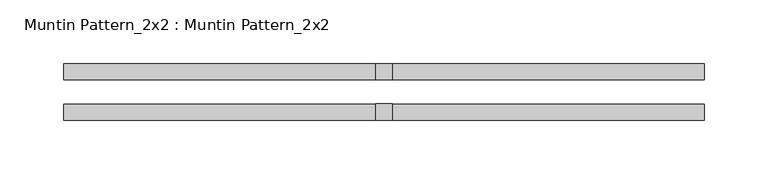
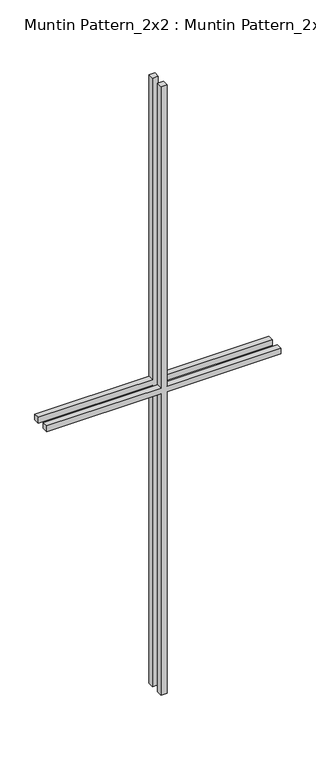
"""IFC4 building model written with IfcOpenShell, lengths in millimetres: proxy geometry, Muntin Pattern_2x2 : Muntin Pattern_2x2."""

from ifc_helpers import new_model, si_unit, frame, origin, place, context, project, spatial, polyline, outline, extrude, source, transform, mapped, element, save


def muntin_pattern_2x2_muntin_pattern_2x2_395d1e8c(model_context):
    return source(origin(), model_context, "Body", "SweptSolid", [
        extrude(outline(polyline([(698.5, -6.35), (698.5, -252.1478294), (685.8, -252.1478294), (685.8, -6.35), (0.0, -6.35), (0.0, 6.35), (685.8, 6.35), (685.8, 252.1478294), (698.5, 252.1478294), (698.5, 6.35), (1384.3, 6.35), (1384.3, -6.35), (698.5, -6.35)])), frame((0.0, 9.525, 0.0), z_axis=(0.0, 1.0, 0.0), x_axis=(0.0, 0.0, 1.0)), (0.0, 0.0, 1.0), 12.7),
        extrude(outline(polyline([(698.5, -6.35), (698.5, -252.1478294), (685.8, -252.1478294), (685.8, -6.35), (0.0, -6.35), (0.0, 6.35), (685.8, 6.35), (685.8, 252.1478294), (698.5, 252.1478294), (698.5, 6.35), (1384.3, 6.35), (1384.3, -6.35), (698.5, -6.35)])), frame((0.0, -22.225, 0.0), z_axis=(0.0, 1.0, 0.0), x_axis=(0.0, 0.0, 1.0)), (0.0, 0.0, 1.0), 12.7),
    ])


if __name__ == "__main__":
    model = new_model("IFC4")
    model_context = context("Model", 3, world=origin())
    ifc_project = project(units=[si_unit("LENGTHUNIT", "METRE", prefix="MILLI")], contexts=[model_context])
    site = spatial("IfcSite", under=ifc_project)
    building = spatial("IfcBuilding", under=site)
    placement = place(None, origin())
    muntin_pattern_2x2_muntin_pattern_2x2_shape = muntin_pattern_2x2_muntin_pattern_2x2_395d1e8c(model_context)
    element("IfcBuildingElementProxy", 1, Name="Muntin Pattern_2x2 : Muntin Pattern_2x2", ObjectType="Muntin Pattern_2x2 : Muntin Pattern_2x2", at=placement, inside=building, context=model_context, shape_type="MappedRepresentation", body=[
        mapped(muntin_pattern_2x2_muntin_pattern_2x2_shape, transform((0.0, 0.0, 0.0), x_axis=(1.0, 0.0, 0.0), y_axis=(0.0, 1.0, 0.0), z_axis=(0.0, 0.0, 1.0))),
    ])
    save(model, "model.ifc")

# Revit data of these elements
# Type "Muntin Pattern_2x2 : Muntin Pattern_2x2"
#   Width [instance default] = 4' - 0"
#   Thickness = 0' - 0 1/2"
#   Height [instance default] = 4' - 0"
#   Distance = 0' - 0 3/4"
#   Interior Material [instance default] = none
#   Exterior Material [instance default] = none
#   Default Elevation = 0
# Element 1 (IfcBuildingElementProxy, "Muntin Pattern_2x2 : Muntin Pattern_2x2")
#   Width = 1' - 7.85416"
#   Height = 4' - 6 1/2"
#   Interior Material = Wood - Stained
#   Exterior Material = Clad - White
#   Materials on its faces: "Clad - White", "Wood - Stained"
# Materials
#   "Clad - White": class "Wood", colour RGB 242 242 238, transparency 0, Cost = 0
#   "Wood - Stained": class "Wood", colour RGB 224 178 126, transparency 0, Cost = 0
